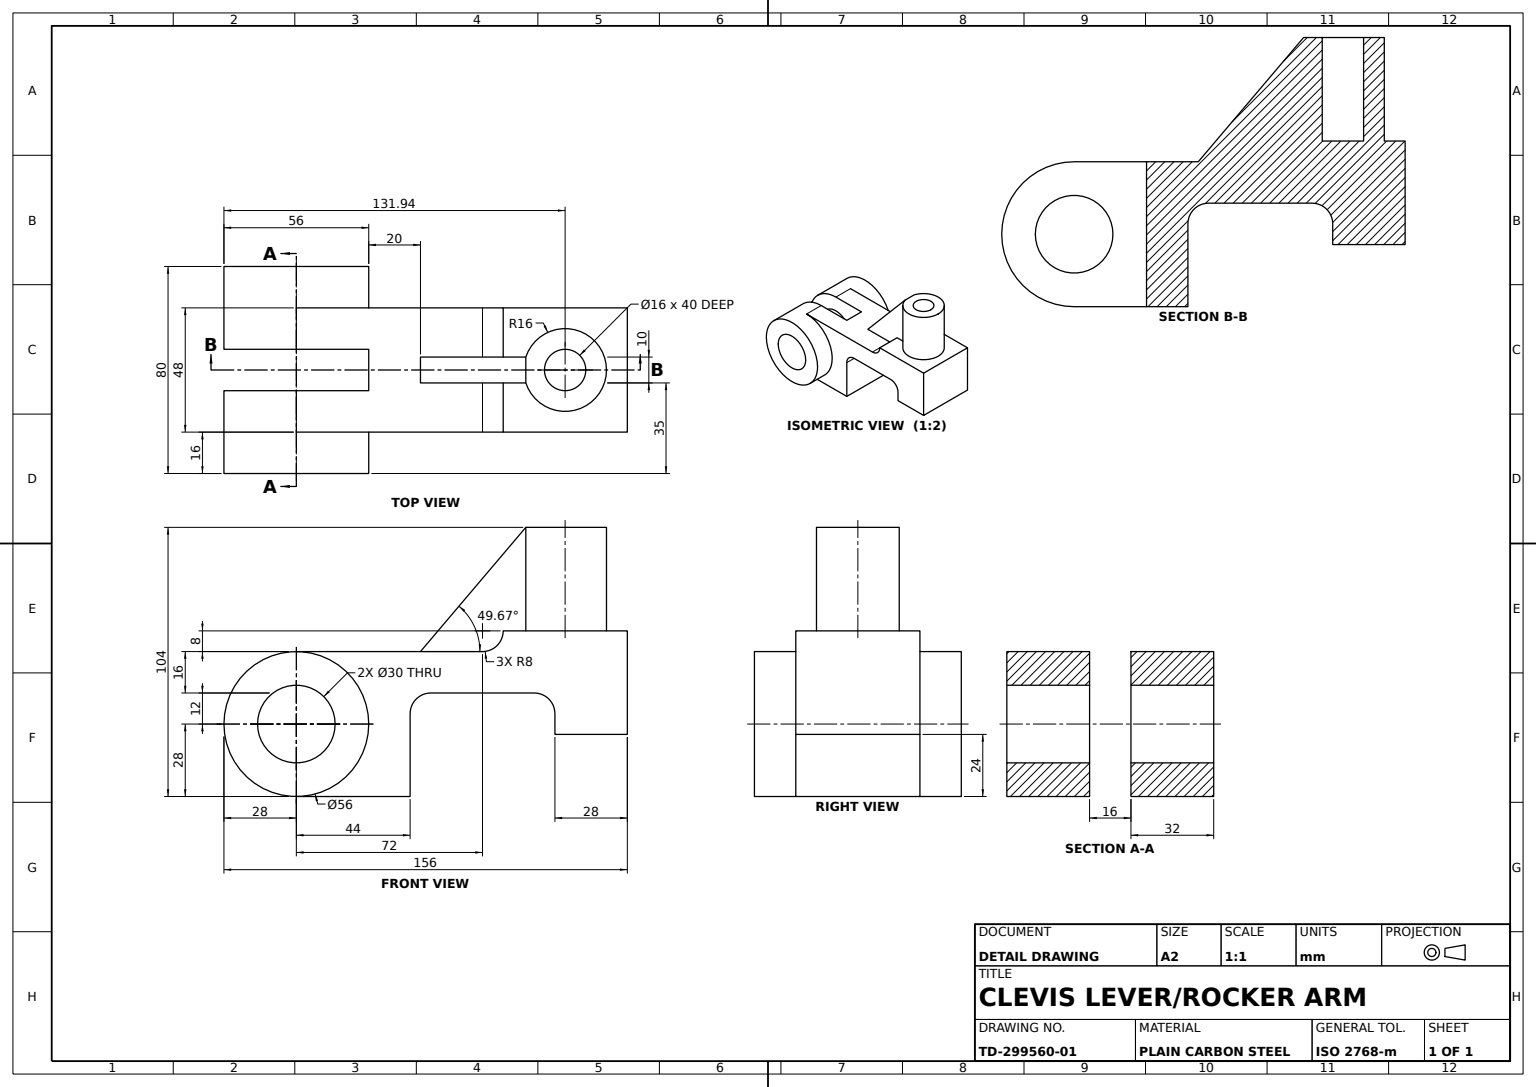
SolidWorks part; units mm, degrees
material "Plain Carbon Steel"
ref_plane "Front Plane" through (0, 0, 0) normal (0, 0, 1) x (1, 0, 0)
ref_plane "Top Plane" through (0, 0, 0) normal (0, 1, 0) x (1, 0, 0)
ref_plane "Right Plane" through (0, 0, 0) normal (1, 0, 0) x (0, 0, -1)
sketch "Pivot Hub Sketch" plane through (0, 0, 0) normal (0, 0, 1) x (1, 0, 0)
  circle A0 centre (0, 0) radius 28
  circle A1 centre (0, 0) radius 15
  dimension "D1" = 56
  dimension "D2" = 30
extrude "Pivot Hub Ø56 Bore Ø30" add sketch "Pivot Hub Sketch" along normal mid plane 80
sketch "Link Arm Profile" plane through (0, 0, 0) normal (0, 0, 1) x (1, 0, 0)
  line L0 (0, 28) -> (72, 28)
  line L1 (80, 36) -> (128, 36)
  line L2 (128, 36) -> (128, -4)
  line L3 (128, -4) -> (100, -4)
  line L4 (100, -4) -> (100, 4)
  line L5 (92, 12) -> (52, 12)
  line L6 (44, 4) -> (44, -28)
  line L7 (44, -28) -> (0, -28)
  circle A0 centre (0, 0) radius 28 construction
  arc A1 (72, 28) -> (80, 36) centre (72, 36) ccw
  arc A2 (100, 4) -> (92, 12) centre (92, 4) ccw
  arc A3 (52, 12) -> (44, 4) centre (52, 4) ccw
  arc A4 (0, -28) -> (0, 28) centre (0, 0) ccw
  dimension "D8" = 8
  dimension "D1" = 16
  dimension "D2" = 24
  dimension "D3" = 40
  dimension "D4" = 72
  dimension "D5" = 56
  dimension "D6" = 56
  dimension "D7" = 28
extrude "Link Arm" add sketch "Link Arm Profile" along normal mid plane 48
sketch "Fork Slot Sketch" plane through (0, 28, 0) normal (0, 1, 0) x (1, 0, 0)
  line L0 (0, -24) -> (0, 24) construction
  line L1 (-35.2475, 8) -> (28, 8)
  line L2 (-35.2475, 8) -> (-35.2475, -8)
  line L3 (-35.2475, -8) -> (28, -8)
  line L4 (28, 8) -> (28, -8)
  point P4 (28, 0)
  dimension "D1" = 16
  dimension "D2" = 28
  dimension "D3" = 35.2475
extrude "Fork Slot 16" cut sketch "Fork Slot Sketch" against normal through all
sketch "Upright Boss Sketch" plane through (0, 36, 0) normal (0, 1, 0) x (1, 0, 0)
  line L0 (80, -24) -> (80, 24) construction
  line L1 (128, 24) -> (80, 24) construction
  circle A0 centre (103.9424, 0) radius 16
  circle A1 centre (103.9424, 0) radius 8
  dimension "D1" = 32
  dimension "D2" = 16
  dimension "D3" = 23.9424
  dimension "D4" = 24
extrude "Upright Boss Ø32 Bore Ø16" add sketch "Upright Boss Sketch" along normal blind 40
sketch "Junction Pad Sketch" plane through (0, 76, 0) normal (0, 1, 0) x (1, 0, 0)
  line L0 (28, -8) -> (28, 8) construction
  line L1 (48, 5) -> (88.7437, 5)
  line L2 (48, 5) -> (48, -5)
  line L3 (48, -5) -> (88.7437, -5)
  circle A0 centre (103.9424, 0) radius 16 construction
  arc A1 (88.7437, 5) -> (88.7437, -5) centre (103.9424, 0) ccw
  point P11 (48, 0)
  dimension "D1" = 20
  dimension "D2" = 10
extrude "Junction Pad" add sketch "Junction Pad Sketch" against normal up to next
sketch "Relief Cut Sketch" plane through (0, 0, 5) normal (0, 0, 1) x (1, 0, 0)
  line L0 (88.7437, 76) -> (48, 28)
  line L1 (48, 76) -> (88.7437, 76) construction
  line L2 (48, 28) -> (48, 76) construction
  line L3 (48, 76) -> (88.7437, 76)
  line L4 (48, 28) -> (48, 76)
extrude "Triangular Relief Cut" cut sketch "Relief Cut Sketch" against normal blind 10
